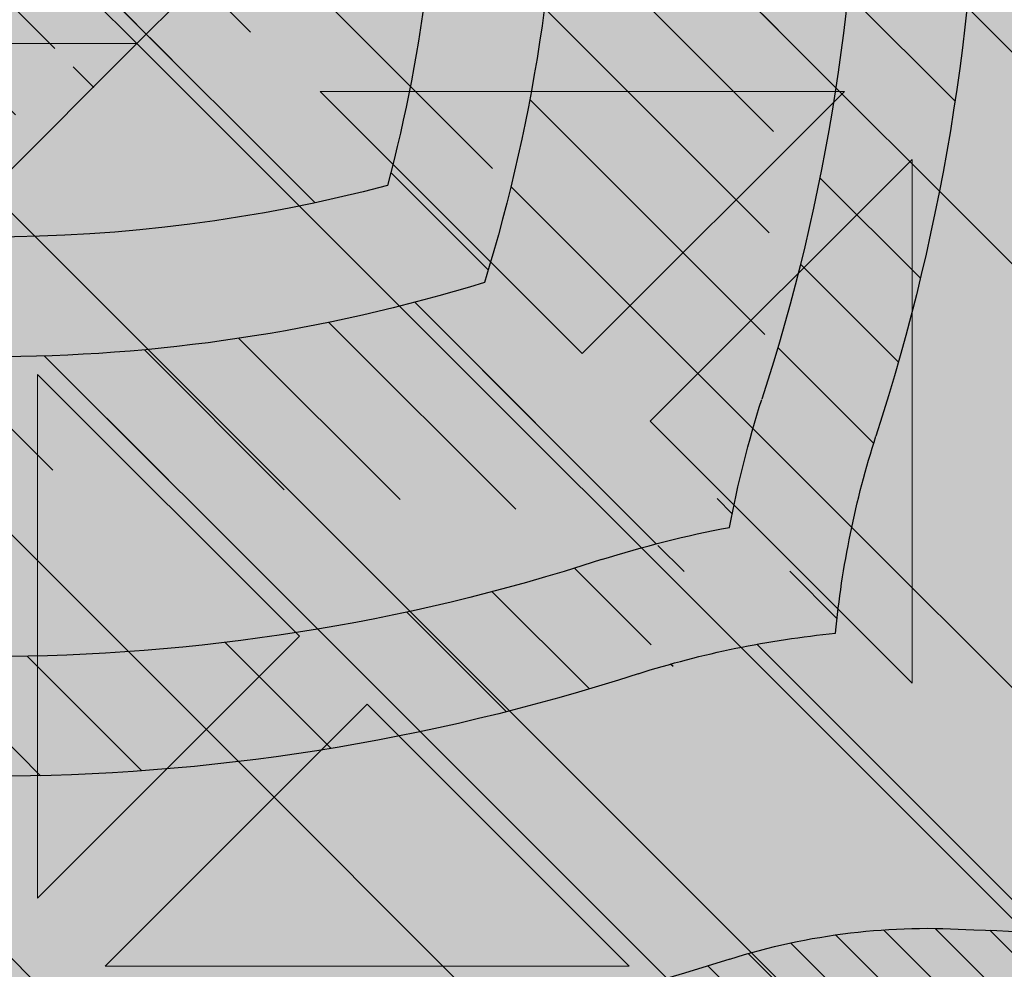
# Model space of a CAD drawing. Units: inches. Extents: x 844 to 2234, y 346 to 1084.
# Tile 28 of 93: x 1257.455 to 1260.074, y 688.657 to 691.183. Entities that reach past the tile are written whole.
import ezdxf

# ---------------------------------------------------------------- set-up
doc = ezdxf.new("R2010")
doc.units = ezdxf.units.IN
doc.header["$MEASUREMENT"] = 0
doc.layers.add('furniture', color=8, linetype='Continuous', lineweight=18)
doc.layers.add('RA-AP-01$0$INT', color=35, linetype='Continuous', lineweight=5)
doc.layers.add('RA-AP-01$0$FURN', color=3, linetype='Continuous')
doc.layers.add('RA-AP-01$0$WOOD', color=64, linetype='Continuous')

# ---------------------------------------------------------------- blocks, each defined once
blk = doc.blocks.new('A$C18D01794')
at = {"layer": 'RA-AP-01$0$INT'}
h = blk.add_hatch(color=256, dxfattribs=at)
h.paths.add_polyline_path([(4.585917135068449, -6.356712009588271), (4.555206456959269, -6.35671200958746), (4.555206456959137, -6.387422687716308), (4.874495778835233, -6.706712009592356), (4.90520645695423, -6.676001331474049)])
h.paths.add_polyline_path([(5.255206456948813, -6.387422687716306), (5.255206456948682, -6.356712009605972), (5.224495778822613, -6.356712009605161), (4.905206456953498, -6.676001331474273), (4.935917135072151, -6.706712009592924)])
h.paths.add_polyline_path([(4.935917135072559, -6.706712009592068), (4.905206456953564, -6.737422687710376), (5.255206456951813, -7.087422687708613), (5.255206456951549, -7.026001331471008)])
h.paths.add_polyline_path([(4.555206456956399, -7.026001331471013), (4.555206456956134, -7.087422687708616), (4.905206456953821, -6.737422687710943), (4.874495778835166, -6.70671200959229)])
h = blk.add_hatch(color=256, dxfattribs=at)
h.paths.add_polyline_path([(4.585917135068448, -6.356712009588273), (4.614201406330596, -6.356712009589021), (4.668846067270487, -6.411356670531338), (4.723490728212344, -6.356712009591912), (4.771774999457151, -6.35671200959319), (4.826419660396886, -6.411356670535356), (4.862780050090322, -6.374996280843536), (4.844495778842715, -6.356712009595112), (4.862780050090411, -6.356712009595595), (4.905206456960182, -6.399138416468211), (4.947632863832445, -6.356712009597838), (4.965917135079675, -6.356712009598322), (4.947632863831759, -6.374996280845421), (4.983993253523576, -6.411356670538857), (5.038637914464627, -6.356712009600247), (5.08692218571208, -6.356712009601523), (5.141566846649976, -6.411356670541852), (5.196211507589851, -6.356712009604411), (5.224495778822615, -6.356712009605161), (4.905206456953975, -6.676001331473793)])
h.paths.add_polyline_path([(4.895206456956031, -6.637717060225675), (4.895206456958921, -6.528427738347902), (4.840561796018589, -6.583072399285802)], flags=16)
h.paths.add_polyline_path([(4.915206456955638, -6.637717060226121), (4.969851117895509, -6.583072399288678), (4.915206456957609, -6.528427738348344)], flags=16)
h.paths.add_polyline_path([(4.826419660395175, -6.568930263661755), (4.881064321335613, -6.514285602723745), (4.771774999456703, -6.514285602720857)], flags=16)
h.paths.add_polyline_path([(4.983993253519558, -6.568930263665262), (5.038637914460456, -6.514285602726792), (4.929348592581548, -6.514285602724816)], flags=16)
h.paths.add_polyline_path([(4.881064321336025, -6.494285602723742), (4.826419660397532, -6.439640941782821), (4.771774999457062, -6.494285602720859)], flags=16)
h.paths.add_polyline_path([(4.929348592582019, -6.494285602724817), (5.038637914460982, -6.494285602726792), (4.983993253522945, -6.439640941786327)], flags=16)
h.paths.add_polyline_path([(4.895206456960191, -6.480143467100443), (4.895206456962115, -6.407422687715913), (4.876922185715016, -6.389138416467584), (4.840561796021581, -6.425498806159401)], flags=16)
h.paths.add_polyline_path([(4.915206456958487, -6.480143467100889), (4.969851117899527, -6.425498806162279), (4.933490728206909, -6.389138416468043), (4.9152064569598, -6.40742268771434)], flags=16)
h.paths.add_polyline_path([(4.757632863832376, -6.480143467096812), (4.812277524772842, -6.425498806158772), (4.757632863834348, -6.370854145217844)], flags=16)
h.paths.add_polyline_path([(4.737632863832376, -6.480143467096286), (4.737632863834348, -6.370854145217375), (4.682988202893906, -6.425498806155385)], flags=16)
h.paths.add_polyline_path([(5.05278005008503, -6.480143467103376), (5.052780050087917, -6.370854145224413), (4.998135389146995, -6.425498806162908)], flags=16)
h.paths.add_polyline_path([(5.072780050085024, -6.480143467103744), (5.127424711025931, -6.42549880616527), (5.072780050087916, -6.370854145224832)], flags=16)
h.paths.add_polyline_path([(4.935917135072783, -6.706712009592292), (5.255206456948811, -6.387422687716309), (5.255206456948932, -6.415706958964177), (5.200561796010279, -6.470351619902839), (5.255206456949403, -6.524996280841948), (5.25520645694961, -6.5732805520894), (5.200561796009787, -6.627925213029239), (5.236922185702417, -6.664285602721864), (5.255206456949919, -6.646001331474357), (5.255206456949998, -6.664285602721898), (5.212780050078687, -6.706712009592262), (5.25520645695036, -6.749138416463932), (5.255206456950438, -6.767422687711313), (5.236922185702424, -6.749138416463297), (5.200561796009796, -6.785498806155928), (5.255206456950753, -6.840143467096874), (5.25520645695096, -6.888427738341682), (5.200561796010322, -6.943072399282328), (5.255206456951428, -6.997717060223427), (5.255206456951547, -7.026001331471006)])
h.paths.add_polyline_path([(5.042988202883395, -6.785498806155427), (5.097632863823085, -6.840143467095101), (5.097632863822622, -6.730854145216193)], flags=16)
h.paths.add_polyline_path([(5.028846067259663, -6.771356670531693), (5.083490728198774, -6.716712009592573), (4.974201406321001, -6.716712009593042)], flags=16)
h.paths.add_polyline_path([(5.117632863823087, -6.840143467095186), (5.172277524762331, -6.785498806155926), (5.11763286382262, -6.730854145216225)], flags=16)
h.paths.add_polyline_path([(5.08349072819877, -6.696712009593886), (5.028846067259652, -6.642067348654775), (4.974201406320998, -6.696712009593438)], flags=16)
h.paths.add_polyline_path([(5.131774999446817, -6.854285602718917), (5.186419660386065, -6.799640941779662), (5.241064321325782, -6.854285602719365)], flags=17)
h.paths.add_polyline_path([(5.131774999446228, -6.716712009592374), (5.186419660386065, -6.771356670532194), (5.222780050079488, -6.734996280838764), (5.204495778832781, -6.716712009592063)], flags=16)
h.paths.add_polyline_path([(5.097632863822613, -6.682569873970264), (5.097632863823061, -6.573280552091354), (5.042988202883383, -6.627925213031044)], flags=16)
h.paths.add_polyline_path([(5.131774999446899, -6.874285602718915), (5.241064321325809, -6.874285602719364), (5.186419660386591, -6.928930263658598)], flags=17)
h.paths.add_polyline_path([(5.131774999446226, -6.696712009594078), (5.204495778830767, -6.696712009594374), (5.22278005007868, -6.67842773834687), (5.186419660386049, -6.642067348654249)], flags=16)
h.paths.add_polyline_path([(5.11763286382262, -6.682569873970225), (5.17227752476232, -6.627925213030515), (5.117632863823064, -6.573280552091267)], flags=16)
h.paths.add_polyline_path([(5.186419660386069, -6.613783077405491), (5.241064321325754, -6.559138416465795), (5.131774999446791, -6.559138416466263)], flags=16)
h.paths.add_polyline_path([(5.131774999446872, -6.539138416466263), (5.24106432132578, -6.539138416465794), (5.186419660386554, -6.484493755526573)], flags=16)
h.paths.add_polyline_path([(5.255206456951811, -7.08742268770861), (5.255206456951895, -7.106712009588038), (4.555206456956052, -7.106712009588038), (4.555206456956136, -7.087422687708617), (4.905206456953973, -6.737422687710788)])
h.paths.add_polyline_path([(4.983993253513404, -6.8444937555241), (4.92934859257295, -6.899138416462108), (5.03863791445186, -6.899138416465014)], flags=16)
h.paths.add_polyline_path([(4.969851117889988, -6.83035161990006), (4.915206456952556, -6.775706958960171), (4.915206456949648, -6.884996280837944)], flags=16)
h.paths.add_polyline_path([(4.929348592572535, -6.919138416462105), (4.983993253511019, -6.973783077403037), (5.038637914451496, -6.919138416465012)], flags=16)
h.paths.add_polyline_path([(5.052780050074912, -6.93328055208906), (4.998135389134438, -6.987925213027088), (5.052780050072919, -7.042569873968025)], flags=16)
h.paths.add_polyline_path([(5.07278005007491, -6.933280552089588), (5.072780050072918, -7.042569873968497), (5.127424711013374, -6.987925213030498)], flags=16)
h.paths.add_polyline_path([(4.89520645695295, -6.775706958959721), (4.840561796013067, -6.830351619897157), (4.895206456950961, -6.884996280837494)], flags=16)
h.paths.add_polyline_path([(4.915206456948365, -6.933280552085403), (4.915206456946434, -7.006001331471951), (4.933490728192729, -7.024285602719066), (4.969851117886972, -6.987925213026453)], flags=16)
h.paths.add_polyline_path([(4.881064321327021, -6.899138416461022), (4.82641966038902, -6.84449375552057), (4.771774999448108, -6.899138416459029)], flags=16)
h.paths.add_polyline_path([(4.895206456950073, -6.933280552084951), (4.840561796009022, -6.987925213023558), (4.876922185700835, -7.024285602716997), (4.895206456948749, -7.006001331469487)], flags=16)
h.paths.add_polyline_path([(4.983993253510392, -7.0020673486505), (4.947632863816944, -7.038427738342319), (4.965917135064043, -7.05671200959023), (5.038637914448995, -7.056712009591555)], flags=16)
h.paths.add_polyline_path([(4.881064321326543, -6.91913841646102), (4.771774999447578, -6.919138416459031), (4.826419660385607, -6.973783077399508)], flags=16)
h.paths.add_polyline_path([(4.905206456946447, -7.014285602717636), (4.862780050074785, -7.056712009588352), (4.947632863816685, -7.056712009589775)], flags=16)
h.paths.add_polyline_path([(5.14156684663679, -7.002067348654549), (5.086922185696452, -7.056712009592438), (5.196211507574223, -7.056712009594425)], flags=16)
h.paths.add_polyline_path([(4.8264196603837, -7.002067348646972), (4.771774999442643, -7.056712009585575), (4.8444957788276, -7.056712009587508), (4.862780050075511, -7.038427738340416)], flags=16)
h.paths.add_polyline_path([(4.812277524760289, -6.98792521302292), (4.757632863822258, -6.933280552082447), (4.757632863819352, -7.042569873961408)], flags=16)
h.paths.add_polyline_path([(4.73763286382226, -6.933280552082079), (4.682988202881349, -6.987925213020536), (4.737632863819352, -7.04256987396099)], flags=16)
h.paths.add_polyline_path([(4.723490728195188, -7.056712009584289), (4.668846067257299, -7.002067348643949), (4.614201406317417, -7.056712009581383)], flags=16)
h.paths.add_polyline_path([(4.597632863829262, -6.706712009592262), (4.555206456957951, -6.664285602721896), (4.555206456958029, -6.646001331474357), (4.573490728205535, -6.664285602721864), (4.609851117898167, -6.627925213029238), (4.555206456958338, -6.573280552089402), (4.555206456958546, -6.524996280841952), (4.60985111789767, -6.470351619902839), (4.555206456959015, -6.415706958964177), (4.555206456959138, -6.387422687716309), (4.874495778835167, -6.70671200959229), (4.5552064569564, -7.026001331471015), (4.555206456956523, -6.997717060223433), (4.609851117897629, -6.94307239928233), (4.555206456956988, -6.888427738341681), (4.555206456957198, -6.840143467096881), (4.609851117898153, -6.78549880615593), (4.573490728205528, -6.749138416463297), (4.555206456957507, -6.76742268771132), (4.555206456957585, -6.749138416463933)])
h.paths.add_polyline_path([(4.712780050085332, -6.730854145216195), (4.712780050084863, -6.840143467095105), (4.767424711024555, -6.785498806155427)], flags=16)
h.paths.add_polyline_path([(4.726922185709173, -6.716712009592573), (4.781566846648288, -6.771356670531693), (4.836211507586949, -6.716712009593043)], flags=16)
h.paths.add_polyline_path([(4.692780050085327, -6.730854145216225), (4.638135389145619, -6.785498806155928), (4.692780050084865, -6.840143467095185)], flags=16)
h.paths.add_polyline_path([(4.726922185709182, -6.696712009593886), (4.836211507586949, -6.696712009593436), (4.7815668466483, -6.642067348654773)], flags=16)
h.paths.add_polyline_path([(4.678637914461726, -6.71671200959237), (4.605917135075169, -6.716712009592063), (4.587632863828464, -6.734996280838766), (4.623993253521887, -6.771356670532195)], flags=16)
h.paths.add_polyline_path([(4.712780050085336, -6.68256987397026), (4.767424711024568, -6.627925213031042), (4.71278005008489, -6.573280552091352)], flags=16)
h.paths.add_polyline_path([(4.678637914461726, -6.696712009594076), (4.623993253521899, -6.642067348654247), (4.587632863829271, -6.67842773834687), (4.605917135077185, -6.696712009594376)], flags=16)
h.paths.add_polyline_path([(4.692780050085336, -6.682569873970228), (4.692780050084889, -6.573280552091267), (4.638135389145632, -6.627925213030515)], flags=16)
h.paths.add_polyline_path([(4.623993253521885, -6.799640941779662), (4.678637914461131, -6.854285602718915), (4.56934859258217, -6.854285602719365)], flags=17)
h.paths.add_polyline_path([(4.623993253521901, -6.613783077405509), (4.678637914461158, -6.559138416466263), (4.569348592582195, -6.559138416465795)], flags=16)
h.paths.add_polyline_path([(4.678637914461051, -6.874285602718915), (4.623993253521361, -6.928930263658598), (4.569348592582143, -6.874285602719364)], flags=17)
h.paths.add_polyline_path([(4.678637914461076, -6.539138416466263), (4.623993253521399, -6.484493755526573), (4.569348592582167, -6.539138416465796)], flags=16)
h = blk.add_hatch(color=256, dxfattribs=at)
h.paths.add_polyline_path([(4.969851117891331, -6.583072399286455), (4.915206456952669, -6.63771706022511), (4.915206456952222, -6.528427738347337)])
h.paths.add_polyline_path([(4.895206456953064, -6.637717060225108), (4.840561796014413, -6.583072399286448), (4.895206456953533, -6.528427738347335)])
h.paths.add_polyline_path([(4.826419660390684, -6.568930263662714), (4.771774999451003, -6.514285602723024), (4.881064321329913, -6.514285602723489)])
h.paths.add_polyline_path([(4.881064321329884, -6.494285602723492), (4.771774999450921, -6.494285602723024), (4.82641966039018, -6.439640941783778)])
h.paths.add_polyline_path([(4.895206456953734, -6.48014346709988), (4.840561796013912, -6.425498806160046), (4.876922185707337, -6.389138416466622), (4.895206456954043, -6.40742268771333)])
h.paths.add_polyline_path([(4.862780050082808, -6.374996280843689), (4.826419660390178, -6.411356670536314), (4.771774999450351, -6.356712009596481), (4.844495778835303, -6.356712009596181)])
h.paths.add_polyline_path([(4.812277524766446, -6.425498806160041), (4.757632863827191, -6.480143467099289), (4.757632863826741, -6.370854145220329)])
h.paths.add_polyline_path([(4.737632863827191, -6.480143467099214), (4.682988202887508, -6.425498806159518), (4.737632863826743, -6.370854145220299)])
h.paths.add_polyline_path([(4.668846067263777, -6.41135667053579), (4.614201406325123, -6.356712009597128), (4.723490728202894, -6.356712009596675)])
h.paths.add_polyline_path([(4.905206456953846, -6.399138416467422), (4.862780050082654, -6.356712009596229), (4.947632863824561, -6.356712009595756)])
h.paths.add_polyline_path([(4.915206456952028, -6.480143467099882), (4.91520645695173, -6.407422687715346), (4.933490728199234, -6.389138416467428), (4.96985111789186, -6.425498806160055)])
h.paths.add_polyline_path([(5.038637914454841, -6.494285602723048), (4.929348592575874, -6.494285602723497), (4.983993253515593, -6.439640941783787)])
h.paths.add_polyline_path([(4.983993253515065, -6.568930263662725), (4.929348592575849, -6.514285602723495), (5.038637914454755, -6.514285602723045)])
h.paths.add_polyline_path([(5.052780050079843, -6.480143467099317), (4.998135389140595, -6.425498806160058), (5.052780050080309, -6.370854145220356)])
h.paths.add_polyline_path([(4.983993253516868, -6.411356670536324), (4.947632863824241, -6.374996280843694), (4.965917135071747, -6.356712009596188), (5.038637914456701, -6.356712009596504)])
h.paths.add_polyline_path([(5.127424711019533, -6.425498806159557), (5.072780050079843, -6.480143467099239), (5.07278005008031, -6.370854145220326)])
h.paths.add_polyline_path([(5.141566846643269, -6.411356670535829), (5.086922185704154, -6.356712009596707), (5.196211507581929, -6.356712009597176)])
h = blk.add_hatch(color=256, dxfattribs=at)
h.paths.add_polyline_path([(4.781566846647504, -6.771356670530272), (4.836211507586161, -6.716712009591613), (4.726922185708388, -6.716712009591159)])
h.paths.add_polyline_path([(4.836211507586161, -6.696712009592008), (4.781566846647504, -6.642067348653354), (4.726922185708388, -6.69671200959247)])
h.paths.add_polyline_path([(4.76742471102377, -6.627925213029623), (4.712780050084083, -6.57328055208994), (4.712780050084542, -6.68256987396885)])
h.paths.add_polyline_path([(4.692780050084544, -6.682569873968819), (4.692780050084084, -6.573280552089856), (4.638135389144834, -6.627925213029111)])
h.paths.add_polyline_path([(4.678637914460932, -6.696712009592669), (4.623993253521102, -6.642067348652844), (4.587632863827676, -6.678427738346266), (4.605917135074382, -6.696712009592973)])
h.paths.add_polyline_path([(4.573490728204743, -6.664285602721736), (4.60985111789737, -6.627925213029108), (4.555206456957541, -6.573280552089279), (4.555206456957237, -6.646001331474231)])
h.paths.add_polyline_path([(4.623993253521098, -6.613783077405377), (4.67863791446035, -6.559138416466126), (4.56934859258139, -6.559138416465669)])
h.paths.add_polyline_path([(4.678637914460275, -6.539138416466126), (4.623993253520583, -6.48449375552644), (4.56934859258136, -6.539138416465672)])
h.paths.add_polyline_path([(4.609851117896854, -6.470351619902707), (4.555206456958196, -6.415706958964051), (4.555206456957738, -6.524996280841822)])
h.paths.add_polyline_path([(4.597632863828475, -6.706712009592775), (4.555206456957283, -6.664285602721582), (4.555206456956805, -6.749138416463489)])
h.paths.add_polyline_path([(4.678637914460932, -6.716712009590963), (4.605917135076396, -6.71671200959066), (4.587632863828479, -6.734996280838164), (4.623993253521104, -6.771356670530792)])
h.paths.add_polyline_path([(4.692780050084091, -6.840143467093776), (4.692780050084548, -6.730854145214809), (4.638135389144834, -6.785498806154524)])
h.paths.add_polyline_path([(4.767424711023772, -6.785498806154004), (4.712780050084545, -6.730854145214786), (4.712780050084089, -6.840143467093692)])
h.paths.add_polyline_path([(4.67863791446036, -6.854285602718778), (4.623993253521105, -6.799640941779527), (4.569348592581399, -6.854285602719237)])
h.paths.add_polyline_path([(4.609851117897371, -6.785498806155798), (4.573490728204743, -6.74913841646317), (4.555206456957237, -6.767422687710675), (4.555206456957548, -6.840143467095629)])
h.paths.add_polyline_path([(4.623993253520596, -6.928930263658465), (4.67863791446028, -6.874285602718778), (4.569348592581367, -6.874285602719238)])
h.paths.add_polyline_path([(4.609851117896867, -6.943072399282199), (4.555206456957749, -6.888427738343082), (4.55520645695821, -6.997717060220857)])
h = blk.add_hatch(color=256, dxfattribs=at)
h.paths.add_polyline_path([(4.905206456953579, -6.70671200959253), (4.905206456953751, -6.676001331474523), (4.874495778835229, -6.706712009592358)])
h.paths.add_polyline_path([(4.935917135071924, -6.706712009592703), (4.905206456953583, -6.706712009592529), (4.90520645695341, -6.737422687710532)])
h = blk.add_hatch(color=256, dxfattribs=at)
h.paths.add_polyline_path([(4.905206456953409, -6.737422687710532), (4.90520645695358, -6.706712009592529), (4.874495778835235, -6.706712009592359)])
h.paths.add_polyline_path([(4.935917135071928, -6.706712009592703), (4.905206456953754, -6.676001331474527), (4.905206456953582, -6.706712009592529)])
for p, q in [((4.905206456953975, -6.676001331473793), (4.585917135071132, -6.356712009590955)), ((4.874495778835167, -6.70671200959229), (4.555206456959136, -6.387422687716307)), ((4.771774999456703, -6.514285602720857), (4.881064321335613, -6.514285602723743)), ((4.826419660395171, -6.568930263661755), (4.771774999456703, -6.514285602720857)), ((4.881064321335613, -6.514285602723743), (4.826419660395173, -6.568930263661757)), ((4.895206456958917, -6.528427738347906), (4.840561796018589, -6.583072399285802)), ((4.895206456958921, -6.528427738347904), (4.895206456956031, -6.637717060225675)), ((4.767424711024566, -6.627925213031041), (4.712780050084888, -6.573280552091352)), ((4.712780050084888, -6.573280552091352), (4.712780050085336, -6.682569873970262)), ((4.895206456956031, -6.637717060225675), (4.840561796018589, -6.583072399285802)), ((4.712780050085336, -6.682569873970262), (4.767424711024568, -6.627925213031042)), ((4.726922185709182, -6.696712009593882), (4.781566846648298, -6.642067348654775)), ((4.836211507586951, -6.696712009593436), (4.781566846648298, -6.642067348654775)), ((4.874495778835233, -6.706712009592356), (4.905206456953753, -6.676001331474525)), ((4.72692218570918, -6.696712009593886), (4.836211507586951, -6.696712009593436)), ((4.874495778835167, -6.70671200959229), (4.555206456956399, -7.026001331471013)), ((4.874495778835233, -6.706712009592356), (4.905206456953409, -6.737422687710532)), ((4.874495778835233, -6.706712009592358), (4.935917135071925, -6.706712009592703))]:
    blk.add_line(p, q, dxfattribs=at)
blk = doc.blocks.new('A$C32926AE1')
at = {"layer": 'RA-AP-01$0$FURN'}
h = blk.add_hatch(dxfattribs=at)
h.set_pattern_fill('ANSI31', color=256, scale=0.1, style=0)
h.set_pattern_definition([(45, (0, 0), (-0.0088388347648318, 0.0088388347648318), [])])
edge = h.paths.add_edge_path(flags=16)
edge.add_arc((4.904771284329206, 4.246793130718756), 0.2603971832811541, 75.22398030683196, 104.7760196931204)
edge.add_arc((4.904771284329206, 4.246793130718756), 0.2603971832811541, 75.223980306832, 104.77601969312039, ccw=False)
edge = h.paths.add_edge_path(flags=16)
edge.add_arc((4.904771284329206, 4.067062675376612), 0.2603971832811541, 255.2239803068796, 284.776019693168)
edge.add_arc((4.904771284329206, 4.067062675376612), 0.2603971832811541, 255.22398030687958, 284.77601969316805, ccw=False)
edge = h.paths.add_edge_path(flags=0)
edge.add_arc((4.904771284329206, 4.067062675376612), 0.2603971832811541, 255.2239803068796, 284.776019693168)
edge.add_arc((4.904771284329206, 4.067062675376612), 0.2603971832811541, 255.22398030687958, 284.77601969316805, ccw=False)
edge = h.paths.add_edge_path(flags=0)
edge.add_arc((4.904771284329206, 4.067062675376612), 0.2603971832811541, 255.2239803068796, 284.776019693168)
edge.add_arc((4.904771284329206, 4.067062675376612), 0.2603971832811541, 255.22398030687958, 284.77601969316805, ccw=False)
edge = h.paths.add_edge_path()
edge.add_arc((4.604388392048174, 4.588829985554312), 0.1599999999999918, 342.3781640246255, 354.4317409793762)
edge.add_arc((5.090145208887507, 4.43216705527679), 0.3503971832811637, 162.0091218307731, 180.3186872093483)
edge.add_arc((5.205154176610243, 4.588829985554953), 0.1599999999999917, 185.5682590208461, 197.6218359767349)
edge.add_arc((4.904771284329229, 4.246793130718735), 0.3503971832811761, 72.00912183053516, 107.9908781690354)
edge.add_arc((9.535952835716557, 4.28682295566602), 4.798342501046485, 178.2875002453811, 181.5576802719453)
edge.add_arc((4.719397359771122, 4.43216705527679), 0.3503971832811637, 359.6813127906516, 377.9908781692269)
edge.add_arc((9.535967292294904, 4.286822350292874), 4.778371420254705, 178.2965938931842, 181.5667745797229)
edge.add_arc((4.719397359771122, 4.43216705527679), 0.3303971832811637, 359.6813127906516, 377.9908781692269)
edge.add_arc((0.2735752763637294, 4.286822350292874), 4.7783714202547, 358.4332254202771, 361.7034061068158)
edge.add_arc((5.061434214606998, 4.732549947558029), 0.1600000000000254, 252.3781640250584, 264.4317409792362)
edge.add_arc((4.748108354051257, 4.732549947558012), 0.1600000000000541, 275.5682590208426, 287.6218359759532)
edge.add_arc((4.604388392048115, 4.588829985554317), 0.1800000000000505, 342.3567572500182, 349.3735009646207)
edge.add_arc((5.205154176610254, 4.588829985554976), 0.1800000000000069, 190.6264990356027, 197.6432427513933)
edge.add_arc((5.061434214607106, 4.732549947558013), 0.1800000000000424, 252.3567572496606, 259.3735009644582)
edge.add_arc((4.904771284329208, 4.246793130718737), 0.3303971832811676, 71.99844483668534, 108.0015551637021)
edge.add_arc((4.748108354051414, 4.732549947558045), 0.1800000000000547, 280.6264990355479, 287.6432427495938)
edge.add_arc((5.090145208887514, 4.432167055276789), 0.2803971832811691, 162.8706300666893, 180.816523289902)
edge.add_arc((4.719397359771136, 4.432167055276689), 0.2803971832811534, 359.183476710103, 377.1293699333214)
edge.add_arc((4.904771284329222, 4.246793130718737), 0.2803971832811769, 72.87063006672916, 107.1293699332334)
edge.add_arc((5.090145208887522, 4.432167055276788), 0.2603971832811776, 165.2239803068007, 180.9953123810312)
edge.add_arc((4.719397359771141, 4.432167055276699), 0.2603971832811458, 359.0046876189768, 374.7760196932087)
edge.add_arc((5.090145208887507, 4.43216705527679), 0.3303971832811637, 162.0091218307731, 180.3186872093483)
edge.add_arc((9.53595427642584, 4.285015535491528), 4.728345371032053, 178.265043920078, 181.5679956281801)
edge.add_arc((0.2735882922327999, 4.285015535491582), 4.728345371032045, 358.4320043718193, 361.7349560799204)
edge.add_arc((9.535953591267507, 4.284458026472751), 4.708343996644348, 178.2573054306777, 181.5704995759608)
edge.add_arc((0.273588977391114, 4.284458026472785), 4.708343996644358, 358.4295004240388, 361.7426945693213)
edge.add_arc((0.2735889773911131, 4.029397779622582), 4.708343996644359, 358.2573054306787, 361.5704995759613)
edge.add_arc((9.535953591267518, 4.029397779622618), 4.708343996644359, 178.4295004240391, 181.7426945693223)
edge.add_arc((0.2735882922327901, 4.028840270603786), 4.728345371032054, 358.2650439200796, 361.5679956281808)
edge.add_arc((9.53595427642584, 4.028840270603841), 4.728345371032054, 178.4320043718199, 181.7349560799219)
edge.add_arc((0.2735752763637302, 4.027033455802493), 4.778371420254699, 358.2965938931842, 361.5667745797229)
edge.add_arc((4.719397359771122, 3.881688750818578), 0.3303971832811637, 342.0091218307731, 360.3186872093484)
edge.add_arc((5.090145208887507, 3.881688750818578), 0.3303971832811637, 179.6813127906516, 197.9908781692269)
edge.add_arc((9.535967292294904, 4.027033455802493), 4.778371420254705, 178.433225420277, 181.7034061068158)
edge.add_arc((4.719397359771122, 3.881688750818578), 0.3503971832811637, 342.0091218307731, 360.3186872093484)
edge.add_arc((9.53595283571655, 4.027032850429349), 4.79834250104648, 178.4423197280546, 181.7124997546188)
edge.add_arc((4.719397359771141, 3.881688750818669), 0.2603971832811458, 345.2239803067913, 360.9953123810232)
edge.add_arc((5.090145208887522, 3.88168875081858), 0.2603971832811776, 179.0046876189687, 194.7760196931993)
edge.add_arc((4.904771284329222, 4.067062675376631), 0.2803971832811769, 252.8706300667665, 287.1293699332708)
edge.add_arc((4.719397359771136, 3.881688750818678), 0.2803971832811534, 342.8706300666787, 360.8165232898969)
edge.add_arc((5.090145208887514, 3.881688750818579), 0.2803971832811691, 179.183476710098, 197.1293699333106)
edge.add_arc((4.748108354051414, 3.581305858537323), 0.1800000000000547, 72.3567572504062, 79.37350096445199)
edge.add_arc((4.904771284329208, 4.067062675376631), 0.3303971832811676, 251.9984448362979, 288.0015551633146)
edge.add_arc((5.061434214607106, 3.581305858537355), 0.1800000000000424, 100.6264990355418, 107.6432427503394)
edge.add_arc((5.205154176610254, 3.725025820540392), 0.1800000000000069, 162.3567572486066, 169.3735009643972)
edge.add_arc((4.604388392048115, 3.725025820541051), 0.1800000000000505, 10.62649903537925, 17.64324274998182)
edge.add_arc((4.748108354051257, 3.581305858537356), 0.1600000000000541, 72.37816402404681, 84.43174097915735)
edge.add_arc((4.904771284329229, 4.067062675376632), 0.3503971832811761, 252.0091218309645, 287.9908781694648)
edge.add_arc((5.061434214606998, 3.581305858537339), 0.1600000000000254, 95.56825902076373, 107.6218359749416)
edge.add_arc((5.205154176610243, 3.725025820540414), 0.1599999999999917, 162.3781640232651, 174.4317409791539)
edge.add_arc((5.090145208887507, 3.881688750818578), 0.3503971832811637, 179.6813127906516, 197.9908781692269)
edge.add_arc((4.604388392048174, 3.725025820541056), 0.1599999999999918, 5.568259020623824, 17.62183597537444)
edge.add_arc((0.2735897329420762, 4.28682295566602), 4.798342501046482, 358.4423197280547, 361.7124997546188)
edge.add_arc((0.2735897329420691, 4.027032850429348), 4.798342501046489, 358.2875002453812, 361.5576802719453)
at = {"layer": 'RA-AP-01$0$WOOD'}
h = blk.add_hatch(color=256, dxfattribs=at)
h.dxf.hatch_style = 1
h.paths.add_polyline_path([(5.157430609644524, 4.573483066760929, -0.1009492694046607), (5.155401577623758, 4.593365984175333, -0.1842662638101597), (5.172249623284174, 4.638795604568598, 0.2056608120311276), (5.179560981299304, 4.661316324430096, 0.3614336704623542), (5.134352340494423, 4.706524965234944, 0.2056608120311297), (5.111831620632933, 4.699213607219793, -0.1842662638101113), (5.066402000239693, 4.682365561559342, -0.1055311479399994), (5.045656153913092, 4.68467289944697, 0.1567636581983829), (4.763886414745334, 4.684672899446966, -0.1055311479399895), (4.743140568418733, 4.68236556155934, -0.1842662638100833), (4.6977109480255, 4.69921360721979, 0.2056608120302612), (4.675190228164109, 4.706524965234949, 0.3614336704708441), (4.629981587358889, 4.66131632442871, 0.2056608120245944), (4.637292945374126, 4.638795604567974, -0.1842662638101024), (4.654140991034615, 4.59336598417475, -0.1009492694055169), (4.652111959013835, 4.573483066760181, 0.021410119221476), (4.629748025606143, 4.156712009541676, 0.0214101192214795), (4.652111959013809, 3.739940952323101, -0.1009492694059586), (4.654140991034615, 3.720058034908448, -0.1842662638100975), (4.637292945374126, 3.674628414515226, 0.2056608120245705), (4.629981587358889, 3.652107694654492, 0.3614336704708879), (4.675190228164113, 3.606899053848249, 0.2056608120302384), (4.697710948025501, 3.614210411863408, -0.1842662638100995), (4.743140568418738, 3.63105845752386, -0.1055311479402541), (4.763886414745388, 3.628751119636215, 0.1567636581983776), (5.045656153913137, 3.628751119636244, -0.1055311479397538), (5.066402000239692, 3.631058457523857, -0.1842662638101067), (5.111831620632931, 3.614210411863407, 0.2056608120310924), (5.134352340494417, 3.606899053848256, 0.3614336704624001), (5.179560981299307, 3.652107694653103, 0.2056608120311314), (5.172249623284175, 3.6746284145146, -0.1842662638101402), (5.155401577623758, 3.72005803490786, -0.1009492694051366), (5.15743060964455, 3.739940952322354, 0.0214101192215073), (5.179794543052287, 4.156712009541468, 0.0214101192215252)])
h.paths.add_polyline_path([(4.639748609479751, 4.156712009541513, 0.0213537860821624), (4.661970494867118, 3.741887061152232, -0.094075836301374), (4.664143710413708, 3.7196126951003, -0.1824818158568985), (4.644813765429836, 3.668037719127816, 0.2056608120245319), (4.639939526753007, 3.653023905887301, 0.3614336704710246), (4.676106439397173, 3.616856993242342, 0.2056608120302234), (4.691120252638095, 3.621731231919122, -0.1824818158602558), (4.742695228611606, 3.641061176902986, -0.1029891339458722), (4.766991894714349, 3.638256818950944, 0.156709409989566), (5.042550673941472, 3.638256818950105, -0.102989133958497), (5.066847340047078, 3.641061176902949, -0.1824818158594995), (5.118422316020358, 3.621731231919103, 0.2056608120311416), (5.133436129261316, 3.616856993242346, 0.3614336704621468), (5.169603041905217, 3.653023905886178, 0.2056608120310986), (5.164728803228477, 3.668037719127177, -0.1824818158565612), (5.145398858244737, 3.719612695099578, -0.0940758363009313), (5.147572073791232, 3.741887061151398, 0.0213537860822023), (5.169793959178681, 4.156712009541451, 0.0213537860822226), (5.147572073791203, 4.571536957931898, -0.0940758363005034), (5.145398858244737, 4.59381132398362, -0.1824818158565587), (5.164728803228476, 4.645386299956021, 0.2056608120311045), (5.169603041905216, 4.66040011319702, 0.3614336704621845), (5.133436129261313, 4.696567025840856, 0.2056608120310773), (5.118422316020359, 4.691692787164098, -0.182481815859508), (5.066847340047078, 4.67236284218025, -0.1029891339584606), (5.04255067394148, 4.675167200133092, 0.156709409989566), (4.766991894714357, 4.675167200132257, -0.1029891339458842), (4.742695228611611, 4.672362842180213, -0.1824818158602725), (4.691120252638095, 4.691692787164077, 0.2056608120302152), (4.676106439397174, 4.696567025840858, 0.3614336704710363), (4.639939526753005, 4.660400113195899, 0.2056608120245495), (4.644813765429837, 4.645386299955384, -0.1824818158568934), (4.664143710413708, 4.593811323982902, -0.0940758363009187), (4.661970494867149, 4.571536957931074, 0.021353786082177)], flags=16)
h.paths.add_polyline_path([(5.129794543052235, 4.432167055276933, -0.0141661062790638), (5.130152669293814, 4.156927903047693, -0.0141661062790647), (5.129794543052234, 3.881688750818433, -0.0785247771143638), (5.10979738006795, 3.755143611847103, 0.0945969212073497), (5.105408519571111, 3.717898134952927, 0.1043170707844957), (5.116074640131521, 3.670385395016088, 0.1043170707864965), (5.068561900193738, 3.681051515576561, 0.09459692119553), (5.031316423304057, 3.676662655080835, -0.1580239521427272), (4.778226145355827, 3.676662655080367, 0.0945969211986668), (4.740980668464973, 3.681051515576592, 0.1043170707882822), (4.693467928526415, 3.670385395015844, 0.1043170707867916), (4.704134049087309, 3.717898134953662, 0.0945969211972894), (4.69974518859162, 3.755143611844042, -0.0785247771163196), (4.679748025606343, 3.881688750818406, -0.0141661062790663), (4.679389899364763, 4.156927903047693, -0.0141661062790672), (4.679748025606343, 4.432167055276998, -0.0785247771163064), (4.699745188591625, 4.55871219425134, 0.094596921197333), (4.704134049087308, 4.595957671141738, 0.1043170707867205), (4.693467928526416, 4.643470411079523, 0.1043170707882628), (4.740980668464965, 4.632804290518776, 0.0945969211988114), (4.778226145355874, 4.637193151015016, -0.158023952142669), (5.031316423304015, 4.637193151014546, 0.0945969211956361), (5.068561900193736, 4.632804290518806, 0.1043170707864979), (5.11607464013152, 4.643470411079278, 0.1043170707844617), (5.105408519571112, 4.595957671142455, 0.0945969212074597), (5.109797380067959, 4.558712194248236, -0.0785247771143467)], flags=0)
h.paths.add_polyline_path([(5.119794532311105, 4.432259799204851, -0.0142000800617244), (5.120156169157484, 4.156927903047701, -0.0142000800617277), (5.119794532311105, 3.881596006890482, -0.0784894509520253), (5.100273383573699, 3.758192358677797, 0.0940138827242913), (5.095413455884425, 3.717477693979438, 0.0606271852308753), (5.099615656341024, 3.686844378806616, 0.0606271852322524), (5.068982341167493, 3.691046579263239, 0.0940138827010453), (5.028267676478798, 3.686186651576848, -0.1580706864508061), (4.781274892180912, 3.686186651576435, 0.0940138827026903), (4.740560227491556, 3.691046579263279, 0.0606271852339895), (4.709926912317155, 3.686844378806508, 0.0606271852329405), (4.714129112773991, 3.717477693980356, 0.094013882701304), (4.709269185087677, 3.758192358669163, -0.0784894509577193), (4.689748036347473, 3.881596006890469, -0.014200080061729), (4.689386399501094, 4.156927903047709, -0.0142000800617217), (4.689748036347473, 4.432259799204808, -0.078489450957724), (4.709269185087651, 4.555663447426125, 0.0940138827014585), (4.714129112773992, 4.596378112114996, 0.0606271852329731), (4.709926912317154, 4.62701142728886, 0.0606271852340196), (4.74056022749157, 4.622809226832087, 0.0940138827024997), (4.781274892180847, 4.627669154518912, -0.1580706864508359), (5.028267676478777, 4.627669154518526, 0.0940138827010946), (5.068982341167492, 4.622809226832129, 0.060627185232254), (5.099615656341024, 4.627011427288751, 0.0606271852308727), (5.095413455884425, 4.59637811211593, 0.0940138827241088), (5.100273383573675, 4.555663447417647, -0.0784894509520978)], flags=0)
h.paths.add_polyline_path([(5.06978912287499, 4.430218106756144, -0.014241683694547), (5.070173729147532, 4.156927903047672, -0.0142416836945458), (5.06978912287499, 3.883637699339223, -0.0800609523125196), (5.052662118612511, 3.773463122773442, 0.0526421978001116), (5.04590916754064, 3.740550867606997, 0.0526421977992423), (5.012996912374707, 3.73379791653534, -0.1583028414718258), (4.796545656286308, 3.73379791653451, 0.0526421978034211), (4.763633401117837, 3.740550867607021, 0.0526421978018622), (4.756880450045755, 3.773463122774558, -0.0800609523117106), (4.739753445783639, 3.883637699339268, -0.0142416836945435), (4.739368839511098, 4.156927903047671, -0.0142416836945477), (4.739753445783639, 4.430218106756155, -0.0800609523116345), (4.75688045004574, 4.540392683320762, 0.052642197801941), (4.763633401117837, 4.573304938488346, 0.0526421978035071), (4.796545656286361, 4.580057889560873, -0.1583028414717561), (5.012996912374669, 4.580057889560039, 0.0526421977993048), (5.04590916754064, 4.57330493848837, 0.0526421978002057), (5.052662118612529, 4.540392683321868, -0.080060952312477)], flags=0)
h.paths.add_polyline_path([(5.049789715110557, 4.43038092723357, -0.0143097550741839), (5.05018085590259, 4.156927903047715, -0.0143097550741854), (5.049789715110558, 3.883474878861827, -0.0800685599149176), (5.03362098255317, 3.779581877367999, 0.0306258898956367), (5.028241146483733, 3.758218888663947, 0.0306258898977031), (5.006878157778253, 3.75283905259408, -0.1583983521624096), (4.802664410878162, 3.752839052594731, 0.0306258898946014), (4.781301422174808, 3.758218888663924, 0.0306258898967912), (4.775921586105202, 3.779581877368794, -0.080068559914251), (4.759752853548071, 3.883474878861786, -0.0143097550741854), (4.759361712756037, 4.156927903047671, -0.0143097550741854), (4.759752853548071, 4.430380927233557, -0.0800685599142479), (4.775921586105193, 4.534273928726546, 0.0306258898968306), (4.781301422174808, 4.555636917431444, 0.0306258898945754), (4.802664410878143, 4.561016753500631, -0.1583983521624168), (5.006878157778244, 4.561016753501291, 0.0306258898977177), (5.028241146483733, 4.555636917431421, 0.0306258898958182), (5.03362098255321, 4.534273928727244, -0.080068559914796)], flags=0)
h.paths.add_polyline_path([(4.999766070382627, 4.428171244713864, -0.0143443147609634), (5.000198441819402, 4.156927903047689, -0.0143443147609612), (4.999766070382627, 3.885684561381556, -0.0784641635803329), (4.987356730658798, 3.799103304488872, -0.1506053783831347), (4.822185837999821, 3.79910330448882, -0.0784641635803318), (4.809776498276007, 3.885684561381509, -0.014344314760963), (4.809344126839227, 4.156927903047677, -0.0143443147609645), (4.809776498276007, 4.428171244713873, -0.0784641635803192), (4.822185837999822, 4.514752501606549, -0.1506053783831338), (4.987356730658798, 4.514752501606494, -0.078464163580285)], flags=0)
h.paths.add_polyline_path([(4.979755254238824, 4.42764379880488, -0.0143772539198268), (4.980205517789977, 4.156927903047693, -0.0143772539198275), (4.979755254238824, 3.886212007290489, -0.0689242507424422), (4.971183264704897, 3.815276770442801, -0.1296645318904179), (4.838359303953726, 3.815276770442746, -0.0689242507424186), (4.829787314419809, 3.886212007290419, -0.0143772539198292), (4.829337050868653, 4.156927903047653, -0.0143772539198325), (4.829787314419809, 4.427643798804946, -0.0689242507424211), (4.838359303953725, 4.498579035652621, -0.1296645318904187), (4.971183264704897, 4.498579035652565, -0.0689242507424401)], flags=0)
h = blk.add_hatch(color=256, dxfattribs=at)
h.dxf.hatch_style = 1
h.paths.add_polyline_path([(5.145398858244737, 4.59381132398362, -0.1824818158565616), (5.164728803228476, 4.645386299956021, 0.2056608120311045), (5.169603041905216, 4.66040011319702, 0.3614336704621845), (5.133436129261313, 4.696567025840856, 0.2056608120310773), (5.118422316020359, 4.691692787164098, -0.182481815859508), (5.066847340047078, 4.67236284218025, -0.1029891339584606), (5.04255067394148, 4.675167200133092, 0.156709409989566), (4.766991894714357, 4.675167200132257, -0.1029891339458842), (4.742695228611611, 4.672362842180213, -0.1824818158602725), (4.691120252638095, 4.691692787164077, 0.2056608120302152), (4.676106439397174, 4.696567025840858, 0.3614336704710363), (4.639939526753005, 4.660400113195899, 0.2056608120245495), (4.644813765429837, 4.645386299955384, -0.1824818158568934), (4.664143710413708, 4.593811323982902, -0.0940758363009187), (4.661970494867149, 4.571536957931074, 0.0213537860821772), (4.639748609479751, 4.156712009541507, 0.0213537860821625), (4.661970494867119, 3.741887061152226, -0.0940758363013071), (4.664143710413708, 3.719612695100309, -0.1824818158569294), (4.644813765429836, 3.668037719127816, 0.2056608120245319), (4.639939526753007, 3.653023905887301, 0.3614336704710246), (4.676106439397173, 3.616856993242342, 0.2056608120302234), (4.691120252638095, 3.621731231919122, -0.1824818158602558), (4.742695228611606, 3.641061176902986, -0.1029891339458722), (4.766991894714349, 3.638256818950944, 0.156709409989566), (5.042550673941472, 3.638256818950105, -0.102989133958497), (5.066847340047078, 3.641061176902949, -0.1824818158594995), (5.118422316020358, 3.621731231919103, 0.2056608120311416), (5.133436129261316, 3.616856993242346, 0.3614336704621468), (5.169603041905217, 3.653023905886178, 0.2056608120310986), (5.164728803228477, 3.668037719127177, -0.1824818158565612), (5.145398858244737, 3.719612695099578, -0.0940758363009313), (5.147572073791232, 3.741887061151398, 0.0213537860822023), (5.169793959178681, 4.156712009541451, 0.0213537860822226), (5.147572073791203, 4.571536957931898, -0.0940758363004996)])
h.paths.add_polyline_path([(5.109797380067958, 4.55871219424824, -0.0785247771143472), (5.129794543052234, 4.432167055276936, -0.0141661062790644), (5.130152669293814, 4.156927903047685, -0.014166106279066), (5.129794543052234, 3.881688750818401, -0.0785247771143517), (5.109797380067946, 3.755143611847092, 0.0945969212073132), (5.105408519571111, 3.717898134952929, 0.1043170707844995), (5.116074640131521, 3.670385395016088, 0.1043170707864965), (5.068561900193738, 3.681051515576561, 0.09459692119553), (5.031316423304057, 3.676662655080835, -0.1580239521427272), (4.778226145355827, 3.676662655080367, 0.0945969211986668), (4.740980668464973, 3.681051515576592, 0.1043170707882822), (4.693467928526415, 3.670385395015844, 0.1043170707867916), (4.704134049087309, 3.717898134953662, 0.0945969211972894), (4.69974518859162, 3.755143611844042, -0.0785247771163196), (4.679748025606343, 3.881688750818406, -0.0141661062790663), (4.679389899364763, 4.156927903047693, -0.0141661062790672), (4.679748025606343, 4.432167055276998, -0.0785247771163064), (4.699745188591625, 4.55871219425134, 0.094596921197333), (4.704134049087308, 4.595957671141738, 0.1043170707867205), (4.693467928526416, 4.643470411079523, 0.1043170707882628), (4.740980668464965, 4.632804290518776, 0.0945969211988114), (4.778226145355874, 4.637193151015016, -0.158023952142669), (5.031316423304015, 4.637193151014546, 0.0945969211956361), (5.068561900193736, 4.632804290518806, 0.1043170707864979), (5.11607464013152, 4.643470411079278, 0.1043170707844617), (5.105408519571112, 4.595957671142455, 0.0945969212074504)], flags=16)
h.paths.add_polyline_path([(5.100273383573655, 4.55566344741771, -0.0784894509521388), (5.119794532311105, 4.432259799204852, -0.0142000800617252), (5.120156169157484, 4.156927903047686, -0.014200080061726), (5.119794532311105, 3.881596006890502, -0.0784894509520446), (5.100273383573696, 3.758192358677786, 0.0940138827242721), (5.095413455884425, 3.717477693979436, 0.0606271852308692), (5.099615656341024, 3.686844378806616, 0.0606271852322522), (5.068982341167493, 3.691046579263239, 0.0940138827010453), (5.028267676478798, 3.686186651576848, -0.1580706864508061), (4.781274892180912, 3.686186651576435, 0.0940138827026903), (4.740560227491556, 3.691046579263279, 0.0606271852339895), (4.709926912317155, 3.686844378806508, 0.0606271852329405), (4.714129112773991, 3.717477693980356, 0.094013882701304), (4.709269185087677, 3.758192358669163, -0.0784894509577193), (4.689748036347473, 3.881596006890469, -0.014200080061729), (4.689386399501094, 4.156927903047709, -0.0142000800617217), (4.689748036347473, 4.432259799204808, -0.078489450957724), (4.709269185087651, 4.555663447426125, 0.0940138827014585), (4.714129112773992, 4.596378112114996, 0.0606271852329731), (4.709926912317154, 4.62701142728886, 0.0606271852340196), (4.74056022749157, 4.622809226832087, 0.0940138827024997), (4.781274892180847, 4.627669154518912, -0.1580706864508359), (5.028267676478777, 4.627669154518526, 0.0940138827010946), (5.068982341167492, 4.622809226832129, 0.060627185232254), (5.099615656341024, 4.627011427288751, 0.0606271852308727), (5.095413455884425, 4.59637811211593, 0.094013882723957)], flags=0)
h.paths.add_polyline_path([(5.04590916754064, 4.57330493848837, 0.0526421978002057), (5.052662118612529, 4.540392683321868, -0.0800609523124783), (5.06978912287499, 4.430218106756142, -0.0142416836945469), (5.070173729147532, 4.156927903047672, -0.0142416836945458), (5.06978912287499, 3.883637699339223, -0.0800609523125196), (5.052662118612511, 3.773463122773442, 0.0526421978001116), (5.04590916754064, 3.740550867606997, 0.0526421977992423), (5.012996912374707, 3.73379791653534, -0.1583028414718258), (4.796545656286308, 3.73379791653451, 0.0526421978034211), (4.763633401117837, 3.740550867607021, 0.0526421978018622), (4.756880450045755, 3.773463122774558, -0.0800609523117106), (4.739753445783639, 3.883637699339268, -0.0142416836945435), (4.739368839511098, 4.156927903047671, -0.0142416836945477), (4.739753445783639, 4.430218106756155, -0.0800609523116345), (4.75688045004574, 4.540392683320762, 0.052642197801941), (4.763633401117837, 4.573304938488346, 0.0526421978035071), (4.796545656286361, 4.580057889560873, -0.1583028414717561), (5.012996912374669, 4.580057889560039, 0.0526421977993048)], flags=0)
h.paths.add_polyline_path([(5.028241146483733, 4.555636917431422, 0.0306258898956949), (5.033620982553182, 4.534273928727329, -0.0800685599148649), (5.049789715110557, 4.430380927233569, -0.0143097550741839), (5.05018085590259, 4.156927903047715, -0.0143097550741854), (5.049789715110558, 3.883474878861827, -0.0800685599149176), (5.03362098255317, 3.779581877367999, 0.0306258898956367), (5.028241146483733, 3.758218888663947, 0.0306258898977031), (5.006878157778253, 3.75283905259408, -0.1583983521624096), (4.802664410878162, 3.752839052594731, 0.0306258898946014), (4.781301422174808, 3.758218888663924, 0.0306258898967912), (4.775921586105202, 3.779581877368794, -0.080068559914251), (4.759752853548071, 3.883474878861786, -0.0143097550741854), (4.759361712756037, 4.156927903047671, -0.0143097550741854), (4.759752853548071, 4.430380927233557, -0.0800685599142479), (4.775921586105193, 4.534273928726546, 0.0306258898968306), (4.781301422174808, 4.555636917431444, 0.0306258898945754), (4.802664410878143, 4.561016753500631, -0.1583983521624168), (5.006878157778244, 4.561016753501291, 0.0306258898977174)], flags=0)
h.paths.add_polyline_path([(4.987356730658798, 4.514752501606494, -0.0784641635803018), (4.999766070382627, 4.428171244713845, -0.0143443147609637), (5.000198441819402, 4.156927903047665, -0.0143443147609622), (4.999766070382628, 3.885684561381514, -0.0784641635802952), (4.987356730658797, 3.799103304488872, -0.1506053783831338), (4.822185837999821, 3.799103304488819, -0.0784641635803342), (4.809776498276007, 3.885684561381512, -0.0143443147609628), (4.809344126839227, 4.156927903047676, -0.0143443147609646), (4.809776498276007, 4.428171244713873, -0.0784641635803192), (4.822185837999822, 4.514752501606549, -0.1506053783831338)], flags=0)
h.paths.add_polyline_path([(4.971183264704897, 4.498579035652566, -0.0689242507424384), (4.979755254238824, 4.427643798804883, -0.0143772539198276), (4.980205517789977, 4.15692790304768, -0.0143772539198258), (4.979755254238823, 3.88621200729051, -0.0689242507424628), (4.971183264704897, 3.815276770442801, -0.129664531890417), (4.838359303953726, 3.815276770442746, -0.0689242507424186), (4.829787314419809, 3.886212007290419, -0.0143772539198292), (4.829337050868653, 4.156927903047653, -0.0143772539198325), (4.829787314419809, 4.427643798804946, -0.0689242507424211), (4.838359303953725, 4.498579035652621, -0.1296645318904187)], flags=0)
h = blk.add_hatch(dxfattribs=at)
h.set_pattern_fill('ANSI31', color=256, scale=0.05, style=0)
h.set_pattern_definition([(45, (0, 0), (-0.0044194173824159, 0.0044194173824159), [])])
h.paths.add_polyline_path([(5.130152669293814, 4.156927903047704, 0.0141661062790657), (5.129794543052234, 4.432167055276982, 0.0777827904001433), (5.110168979996553, 4.557559993161921, -0.0976515123401879), (5.105408519571111, 4.595957671142454, -0.1043170707844687), (5.116074640131522, 4.64347041107928), (5.099615656341024, 4.627011427288751, 0.0606271852308727), (5.095413455884425, 4.59637811211593, 0.0940138827241088), (5.100273383573675, 4.555663447417647, -0.0784894509520972), (5.119794532311105, 4.432259799204852, -0.0142000800617252), (5.120156169157484, 4.156927903047686, -0.014200080061726), (5.119794532311105, 3.881596006890502, -0.0784894509520446), (5.100273383573696, 3.758192358677786, 0.0940138827242721), (5.095413455884425, 3.717477693979436, 0.0606271852308692), (5.099615656341024, 3.686844378806616), (5.116074640131519, 3.67038539501609, -0.1043170707844594), (5.105408519571112, 3.717898134952912, -0.0976515123401594), (5.11016897999655, 3.756295812933435, 0.0777827904001654), (5.129794543052234, 3.881688750818409, 0.0141661062790665)])
h.paths.add_polyline_path([(5.030164222210597, 3.676291055149937, -0.0976515123472002), (5.068561900193739, 3.681051515576561, -0.1043170707864927), (5.116074640131521, 3.670385395016088), (5.099615656341024, 3.686844378806616, 0.0606271852322522), (5.068982341167493, 3.691046579263239, 0.0940138827010453), (5.028267676478798, 3.686186651576848, -0.1580706864508061), (4.781274892180912, 3.686186651576435, 0.0940138827026903), (4.740560227491556, 3.691046579263279, 0.0606271852339913), (4.709926912317154, 3.686844378806508), (4.693467928526416, 3.670385395015845, -0.1043170707882796), (4.740980668464973, 3.681051515576592, -0.0976515123427246), (4.779378346446416, 3.676291055150394, 0.156512506893803)])
h.paths.add_polyline_path([(4.689748036347473, 3.881596006890472, -0.014200080061729), (4.689386399501094, 4.156927903047712, -0.0142000800617195), (4.689748036347473, 4.432259799204768, -0.078489450957742), (4.709269185087648, 4.555663447426114, 0.0940138827014821), (4.714129112773992, 4.596378112114995, 0.0606271852329748), (4.709926912317154, 4.62701142728886), (4.693467928526414, 4.643470411079524, -0.1043170707867939), (4.704134049087309, 4.595957671141706, -0.09765151234893), (4.699373588660725, 4.557559993157876, 0.0777827903975372), (4.679748025606343, 4.432167055276987, 0.0141661062790675), (4.679389899364763, 4.156927903047675, 0.0141661062790641), (4.679748025606343, 3.88168875081843, 0.0777827903975637), (4.699373588660724, 3.756295812937497, -0.0976515123490278), (4.704134049087308, 3.717898134953629, -0.1043170707867196), (4.693467928526416, 3.670385395015845), (4.709926912317155, 3.686844378806508, 0.0606271852329413), (4.714129112773991, 3.717477693980357, 0.0940138827013084), (4.709269185087676, 3.758192358669166, -0.0784894509577192)])
h.paths.add_polyline_path([(4.779378346446434, 4.63756475094498, -0.0976515123427943), (4.740980668464964, 4.632804290518776, -0.1043170707882609), (4.693467928526416, 4.643470411079523), (4.709926912317154, 4.62701142728886, 0.0606271852340196), (4.74056022749157, 4.622809226832087, 0.0940138827024997), (4.781274892180847, 4.627669154518912, -0.1580706864508359), (5.028267676478777, 4.627669154518526, 0.0940138827010946), (5.068982341167492, 4.622809226832129, 0.060627185232254), (5.099615656341024, 4.627011427288751), (5.116074640131521, 4.643470411079279, -0.1043170707865022), (5.068561900193735, 4.632804290518806, -0.0976515123475899), (5.030164222210446, 4.637564750945479, 0.1565125068936924)])
h = blk.add_hatch(dxfattribs=at)
h.set_pattern_fill('ANSI32', color=256, scale=0.2, style=0)
h.set_pattern_definition([(45, (0, 0), (-0.0530330085889911, 0.0530330085889911), []), (45, (0.035355339, 0), (-0.0530330085889911, 0.0530330085889911), [])])
h.paths.add_polyline_path([(5.119794532311105, 4.432259799204823, 0.0777015974868765), (5.10065834347252, 4.554469821747928, -0.0968902511992216), (5.095413455884425, 4.596378112115931, -0.060627185230871), (5.099615656341024, 4.627011427288751, -0.060627185232254), (5.068982341167492, 4.622809226832129, -0.0968902512198245), (5.027074050790956, 4.628054114423209, 0.1564657949319105), (4.782468517866163, 4.628054114422785, -0.0968902512152247), (4.740560227491555, 4.622809226832088, -0.0606271852339878), (4.709926912317155, 4.627011427288859, -0.0606271852329413), (4.714129112773991, 4.596378112115011, -0.0968902512205338), (4.708884225182929, 4.554469821738175, 0.0777015974804443), (4.689748036347473, 4.43225979920482, 0.0142000800617215), (4.689386399501094, 4.156927903047726, 0.0142000800617273), (4.689748036347473, 3.88159600689052, 0.077701597480541), (4.708884225182985, 3.759385984357019, -0.096890251220082), (4.714129112773992, 3.717477693980371, -0.0606271852329731), (4.709926912317154, 3.686844378806507, -0.060627185233988), (4.740560227491554, 3.691046579263279, -0.0968902512152569), (4.782468517866175, 3.685801691672578, 0.1564657949319236), (5.027074050790988, 3.685801691672169, -0.0968902512197451), (5.068982341167491, 3.691046579263239, -0.0606271852322557), (5.099615656341024, 3.686844378806616, -0.0606271852308727), (5.095413455884425, 3.717477693979438, -0.0968902511991229), (5.100658343472507, 3.7593859843474, 0.0777015974868745), (5.119794532311105, 3.8815960068905, 0.014200080061726), (5.120156169157484, 4.156927903047685, 0.0142000800617238)])
h.paths.add_polyline_path([(5.070173729147531, 4.156927903047684, -0.0142416836945481), (5.06978912287499, 3.883637699339191, -0.0800609523125107), (5.052662118612505, 3.773463122773424, 0.0526421978000811), (5.04590916754064, 3.740550867606997, 0.0526421977993214), (5.012996912374658, 3.733797916535325, -0.1583028414717916), (4.796545656286304, 3.733797916534512, 0.0526421978034138), (4.763633401117837, 3.740550867607021, 0.0526421978018622), (4.756880450045755, 3.773463122774558, -0.0800609523117106), (4.739753445783639, 3.883637699339268, -0.0142416836945435), (4.739368839511098, 4.156927903047671, -0.0142416836945477), (4.739753445783639, 4.430218106756155, -0.0800609523116345), (4.75688045004574, 4.540392683320762, 0.052642197801941), (4.763633401117837, 4.573304938488346, 0.0526421978035071), (4.796545656286361, 4.580057889560873, -0.1583028414717561), (5.012996912374669, 4.580057889560039, 0.0526421977993048), (5.04590916754064, 4.57330493848837, 0.0526421978002057), (5.052662118612529, 4.540392683321868, -0.0800609523124783), (5.06978912287499, 4.430218106756142, -0.0142416836945463)], flags=16)
h.paths.add_polyline_path([(5.050180855902591, 4.156927903047686, -0.0143097550741856), (5.049789715110558, 3.883474878861795, -0.0800685599148126), (5.033620982553202, 3.7795818773681, 0.0306258898957837), (5.028241146483733, 3.758218888663947, 0.0306258898977031), (5.006878157778253, 3.75283905259408, -0.1583983521624096), (4.802664410878162, 3.752839052594731, 0.0306258898946014), (4.781301422174808, 3.758218888663924, 0.0306258898967912), (4.775921586105202, 3.779581877368794, -0.080068559914251), (4.759752853548071, 3.883474878861786, -0.0143097550741854), (4.759361712756037, 4.156927903047671, -0.0143097550741854), (4.759752853548071, 4.430380927233557, -0.0800685599142479), (4.775921586105193, 4.534273928726546, 0.0306258898968306), (4.781301422174808, 4.555636917431444, 0.0306258898945754), (4.802664410878143, 4.561016753500631, -0.1583983521624168), (5.006878157778244, 4.561016753501291, 0.0306258898977177), (5.028241146483733, 4.555636917431421, 0.0306258898958182), (5.03362098255321, 4.534273928727244, -0.0800685599147973), (5.049789715110557, 4.430380927233568, -0.0143097550741854)], flags=0)
h.paths.add_polyline_path([(5.000198441819402, 4.15692790304769, -0.0143443147609622), (4.999766070382627, 3.885684561381539, -0.0784641635803169), (4.987356730658798, 3.799103304488873, -0.1506053783831347), (4.822185837999821, 3.79910330448882, -0.0784641635803318), (4.809776498276007, 3.885684561381509, -0.014344314760963), (4.809344126839227, 4.156927903047677, -0.0143443147609645), (4.809776498276007, 4.428171244713873, -0.0784641635803192), (4.822185837999822, 4.514752501606549, -0.1506053783831338), (4.987356730658798, 4.514752501606494, -0.0784641635803018), (4.999766070382627, 4.428171244713845, -0.0143443147609624)], flags=0)
h.paths.add_polyline_path([(4.980205517789976, 4.156927903047707, -0.0143772539198295), (4.979755254238824, 3.886212007290466, -0.06892425074242), (4.971183264704897, 3.815276770442801, -0.129664531890417), (4.838359303953726, 3.815276770442746, -0.0689242507424186), (4.829787314419809, 3.886212007290419, -0.0143772539198292), (4.829337050868653, 4.156927903047653, -0.0143772539198325), (4.829787314419809, 4.427643798804946, -0.0689242507424211), (4.838359303953725, 4.498579035652621, -0.1296645318904187), (4.971183264704897, 4.498579035652565, -0.0689242507424418), (4.979755254238824, 4.427643798804878, -0.0143772539198259)], flags=0)
for centre, radius, start, end in [((5.090145208887514, 3.881688750818579), 0.2803971832811691, 179.183476710098, 197.1293699333106), ((5.090145208887522, 3.88168875081858), 0.2603971832811776, 179.0046876189687, 194.7760196931993), ((5.090145208887507, 3.881688750818578), 0.3503971832811637, 179.6813127906516, 197.9908781692269), ((5.090145208887507, 3.881688750818578), 0.3303971832811637, 179.6813127906516, 197.9908781692269), ((4.904771284329206, 4.067062675376612), 0.2603971832811541, 255.2239803068796, 284.776019693168), ((4.904771284329206, 4.067062675376612), 0.2603971832811541, 255.2239803068796, 284.776019693168), ((4.904771284329222, 4.067062675376631), 0.2803971832811769, 252.8706300667665, 287.1293699332708), ((4.604388392048115, 3.725025820541051), 0.1800000000000505, 10.62649903537925, 17.64324274998182), ((4.604388392048174, 3.725025820541056), 0.1599999999999918, 5.568259020623824, 17.62183597537444), ((4.748108354051414, 3.581305858537323), 0.1800000000000547, 72.3567572504062, 79.37350096445199), ((4.904771284329208, 4.067062675376631), 0.3303971832811676, 251.9984448362979, 288.0015551633146), ((4.748108354051257, 3.581305858537356), 0.1600000000000541, 72.37816402404681, 84.43174097915735), ((4.904771284329229, 4.067062675376632), 0.3503971832811761, 252.0091218309645, 287.9908781694648), ((4.748108354051327, 3.581305858537359), 0.1100000000000303, 72.45144083744763, 93.9346900888063), ((4.742507915094622, 3.563091385939261), 0.1279700159630606, 90.8720682532012, 104.749808972944), ((4.904771284329219, 4.067062675376634), 0.4003971832811741, 252.0350753990311, 287.9649246011635)]:
    blk.add_arc(centre, radius, start, end, dxfattribs=at)
blk = doc.blocks.new('A$C5D2F253E')
at = {"layer": 'RA-AP-01$0$FURN', "xscale": -0.7999999999883585, "yscale": 0.7999999999883585, "zscale": 0.8, "rotation": 90}
blk.add_blockref('A$C18D01794', (-5.687757199772477, 4.75791982714071), dxfattribs=at)
at = {"layer": 'RA-AP-01$0$WOOD', "rotation": 270}
blk.add_blockref('A$C32926AE1', (-4.161339601644158, 5.73852594588169), dxfattribs=at)

msp = doc.modelspace()

# ---------------------------------------------------------------- block references
at = {"layer": 'furniture', "xscale": -15.94108302203742, "yscale": 15.94108302203742, "zscale": 15.94108302203742, "rotation": 270}
msp.add_blockref('A$C5D2F253E', (1244.08405109492, 696.2584716700112), dxfattribs=at)

doc.saveas('drawing.dxf')
